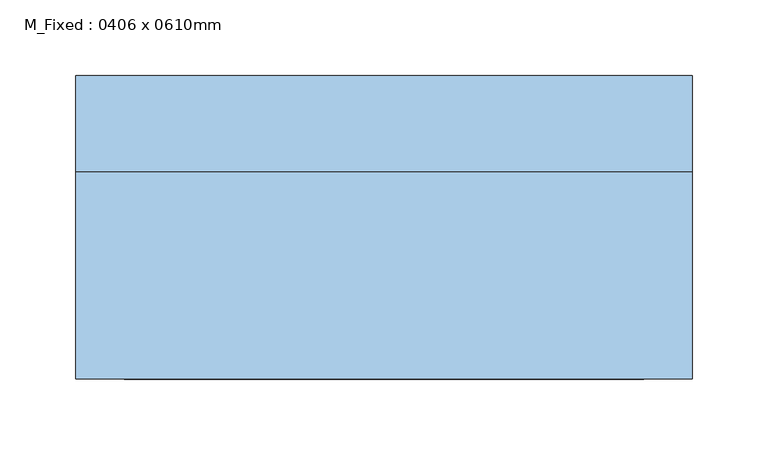
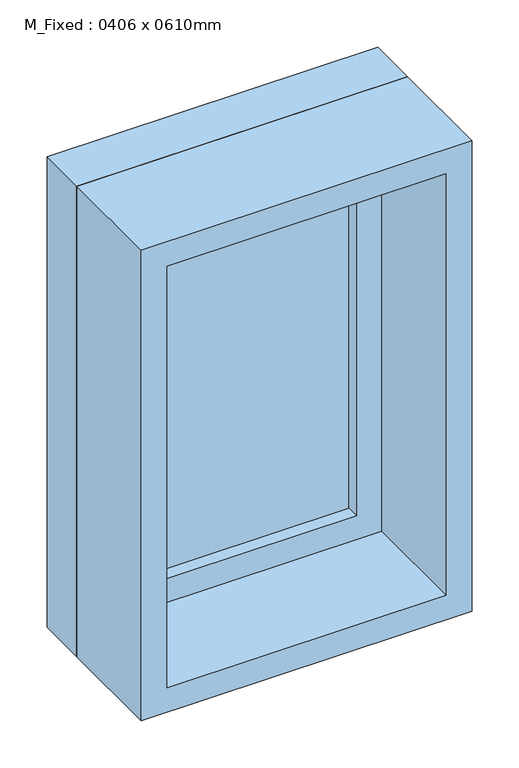
"""IFC4 building model written with IfcOpenShell, lengths in millimetres: window geometry, M_Fixed : 0406 x 0610mm."""

from ifc_helpers import new_model, si_unit, frame, origin, place, context, project, spatial, polyline, outline, extrude, source, transform, mapped, element, save


def m_fixed_0406_x_0610mm_8205b201(model_context):
    return source(origin(), model_context, "Body", "SweptSolid", [
        extrude(outline(polyline([(-140.0, 78.0), (140.0, 78.0), (140.0, 66.0), (-140.0, 66.0), (-140.0, 78.0)])), frame((0.0, 0.0, 978.0), z_axis=(0.0, 0.0, 1.0), x_axis=(1.0, 0.0, 0.0)), (0.0, 0.0, 1.0), 484.0),
        extrude(outline(polyline([(1506.0, -184.0), (934.0, -184.0), (934.0, 184.0), (1506.0, 184.0), (1506.0, -184.0)]), holes=[polyline([(1462.0, -140.0), (1462.0, 140.0), (978.0, 140.0), (978.0, -140.0), (1462.0, -140.0)])]), frame((0.0, 50.0, 0.0), z_axis=(0.0, 1.0, 0.0), x_axis=(0.0, 0.0, 1.0)), (0.0, 0.0, 1.0), 44.0),
        extrude(outline(polyline([(1525.0, -203.0), (915.0, -203.0), (915.0, 203.0), (1525.0, 203.0), (1525.0, -203.0)]), holes=[polyline([(1506.0, -184.0), (1506.0, 184.0), (934.0, 184.0), (934.0, -184.0), (1506.0, -184.0)])]), frame((0.0, 50.0, 0.0), z_axis=(0.0, 1.0, 0.0), x_axis=(0.0, 0.0, 1.0)), (0.0, 0.0, 1.0), 63.0),
        extrude(outline(polyline([(1525.0, -203.0), (915.0, -203.0), (915.0, 203.0), (1525.0, 203.0), (1525.0, -203.0)]), holes=[polyline([(1493.0, -171.0), (1493.0, 171.0), (947.0, 171.0), (947.0, -171.0), (1493.0, -171.0)])]), frame((0.0, -87.0, 0.0), z_axis=(0.0, 1.0, 0.0), x_axis=(0.0, 0.0, 1.0)), (0.0, 0.0, 1.0), 137.0),
    ])


if __name__ == "__main__":
    model = new_model("IFC4")
    model_context = context("Model", 3, world=origin())
    ifc_project = project(units=[si_unit("LENGTHUNIT", "METRE", prefix="MILLI")], contexts=[model_context])
    site = spatial("IfcSite", under=ifc_project)
    building = spatial("IfcBuilding", under=site)
    placement = place(None, origin())
    m_fixed_0406_x_0610mm_shape = m_fixed_0406_x_0610mm_8205b201(model_context)
    element("IfcWindow", 1, ObjectType="M_Fixed : 0406 x 0610mm", at=placement, inside=building, context=model_context, shape_type="MappedRepresentation", body=[
        mapped(m_fixed_0406_x_0610mm_shape, transform((0.0, 0.0, 0.0), x_axis=(1.0, 0.0, 0.0), y_axis=(0.0, 1.0, 0.0), z_axis=(0.0, 0.0, 1.0))),
    ])
    save(model, "model.ifc")

# Revit data of these elements
# Type "M_Fixed : 0406 x 0610mm"
#   Type Mark = "10"
#   Height = 2' - 0.01575"
#   Default Sill Height = 3' - 0.02362"
#   Width = 1' - 3.98425"
#   Window Inset = 0' - 0.74803"
#   Frame Exterior Material = Sash
#   Frame Interior Material = Sash
#   Glass Pane Material = Glass
#   Sash = Sash
#   Wall Closure = (empty or 0)
# Element 1 (IfcWindow, "M_Fixed : 0406 x 0610mm")
#   Materials on its faces: "Sash", "Glass"
# Materials
#   "Sash": class "Wood", colour RGB 136 99 55, transparency 0
#   "Glass": class "Glass", colour RGB 218 227 224, transparency 0.85, Description = "Soda Lime Glass", Cost = 0
